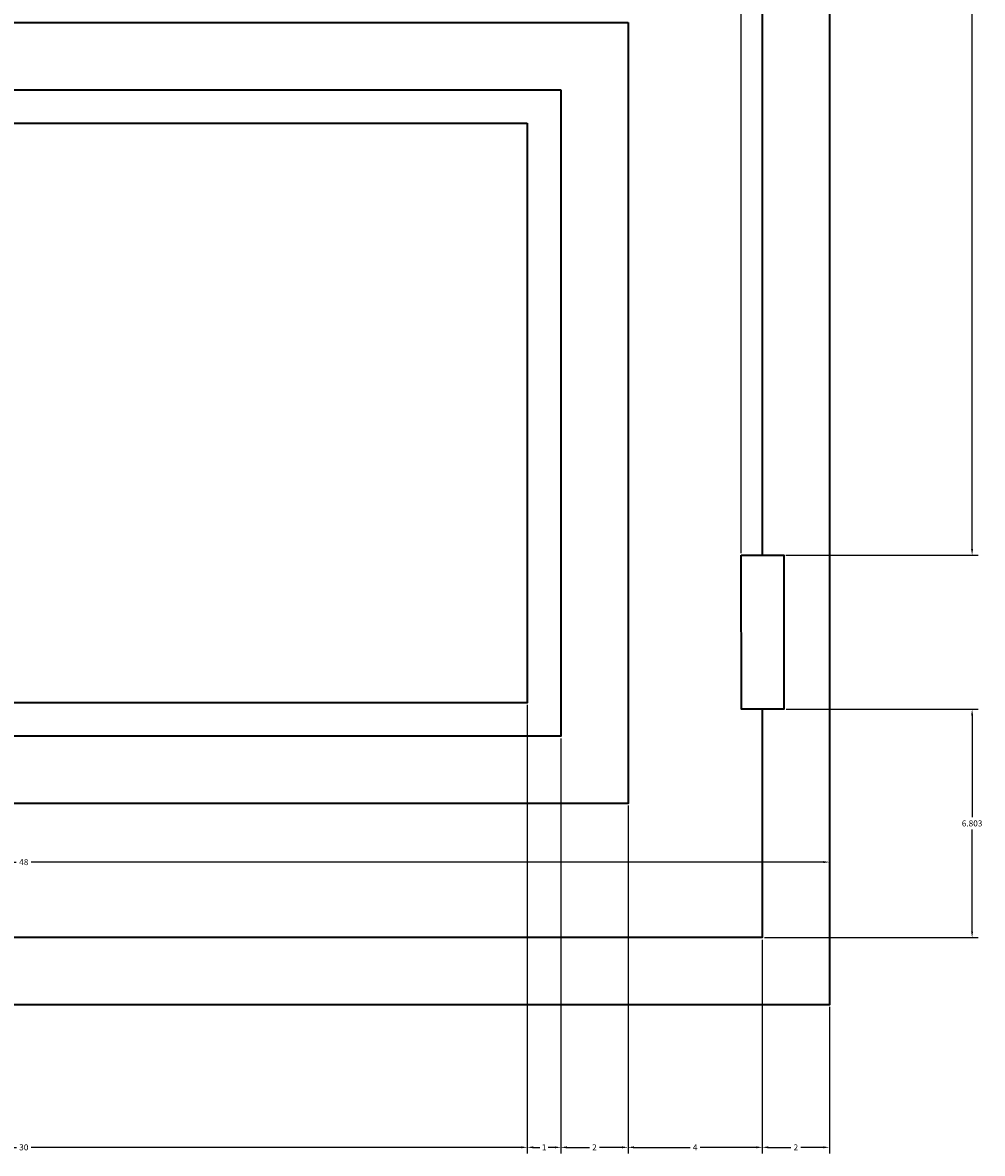
# Model space of a CAD drawing. Units: inches. Extents: x 3137 to 3299, y 1994 to 2089.
# Tile 2 of 14: x 3165 to 3194, y 1994 to 2028. Entities that reach past the tile are written whole.
import ezdxf

# ---------------------------------------------------------------- set-up
doc = ezdxf.new("R2010")
doc.units = ezdxf.units.IN
doc.header["$MEASUREMENT"] = 0
doc.layers.add('A-ANNO-DIMS', color=2, linetype='Continuous', lineweight=18)
doc.layers.add('A-DOOR', color=4, linetype='Continuous', lineweight=35)
doc.styles.get("Standard").update_dxf_attribs({"font": 'arial.ttf'})
doc.dimstyles.get("Standard").update_dxf_attribs({"dimtxt": 0.18, "dimasz": 0.18, "dimexe": 0.18, "dimexo": 0.0625, "dimgap": 0.09, "dimtad": 0, "dimtih": 1, "dimtoh": 1, "dimdec": 4, "dimzin": 0, "dimdsep": 46, "dimtxsty": 'Standard', "dimcen": 0.09, "dimadec": 0, "dimazin": 0, "dimtfac": 1, "dimtdec": 4, "dimtofl": 0, "dimtmove": 0, "dimatfit": 3, "dimfxl": 1, "dimtolj": 1, "dimtzin": 0, "dimarcsym": 0})

# ---------------------------------------------------------------- blocks, each defined once
blk = doc.blocks.new('DOOR-HINGE')
blk.add_lwpolyline([(0, 4.592), (1.268, 4.592), (1.275, 0), (0.007, 0)], close=True)
blk = doc.blocks.new('*D13')
at = {"layer": 'A-ANNO-DIMS', "color": 0, "lineweight": -2, "transparency": 16777216}
for p, q in [((3141.478, 1998.936), (3141.478, 2003.304)), ((3141.658, 2003.124), (3165.255, 2003.124)), ((3189.298, 2003.124), (3165.7, 2003.124)), ((3189.478, 1998.936), (3189.478, 2003.304))]:
    blk.add_line(p, q, dxfattribs=at)
at = {"layer": 'A-ANNO-DIMS', "color": 0, "transparency": 16777216}
for points in [[(3141.658, 2003.154), (3141.658, 2003.094), (3141.478, 2003.124)], [(3189.298, 2003.154), (3189.298, 2003.094), (3189.478, 2003.124)]]:
    blk.add_solid(points, dxfattribs=at)
at = {"layer": 'Defpoints', "color": 0, "transparency": 16777216}
for p in [(3189.478, 2003.124), (3141.478, 1998.874), (3189.478, 1998.874)]:
    blk.add_point(p, dxfattribs=at)
at = {"layer": 'A-ANNO-DIMS', "color": 0, "transparency": 16777216, "insert": (3165.478, 2003.124), "char_height": 0.18, "attachment_point": 5}
blk.add_mtext('\\A1;48', dxfattribs=at)
blk = doc.blocks.new('*D18')
at = {"layer": 'A-ANNO-DIMS', "color": 0, "lineweight": -2, "transparency": 16777216}
for p, q in [((3150.478, 2007.811), (3150.478, 1994.444)), ((3180.478, 2007.811), (3180.478, 1994.444)), ((3150.658, 1994.624), (3165.259, 1994.624)), ((3180.298, 1994.624), (3165.696, 1994.624))]:
    blk.add_line(p, q, dxfattribs=at)
at = {"layer": 'A-ANNO-DIMS', "color": 0, "transparency": 16777216}
for points in [[(3150.658, 1994.654), (3150.658, 1994.594), (3150.478, 1994.624)], [(3180.298, 1994.654), (3180.298, 1994.594), (3180.478, 1994.624)]]:
    blk.add_solid(points, dxfattribs=at)
at = {"layer": 'Defpoints', "color": 0, "transparency": 16777216}
for p in [(3150.478, 2007.874), (3180.478, 2007.874), (3180.478, 1994.624)]:
    blk.add_point(p, dxfattribs=at)
at = {"layer": 'A-ANNO-DIMS', "color": 0, "transparency": 16777216, "insert": (3165.478, 1994.624), "char_height": 0.18, "attachment_point": 5}
blk.add_mtext('\\A1;30', dxfattribs=at)
blk = doc.blocks.new('*D19')
at = {"layer": 'A-ANNO-DIMS', "color": 0, "lineweight": -2, "transparency": 16777216}
for p, q in [((3180.478, 2007.811), (3180.478, 1994.444)), ((3181.478, 2006.811), (3181.478, 1994.444)), ((3180.658, 1994.624), (3180.855, 1994.624)), ((3181.298, 1994.624), (3181.101, 1994.624))]:
    blk.add_line(p, q, dxfattribs=at)
at = {"layer": 'A-ANNO-DIMS', "color": 0, "transparency": 16777216}
for points in [[(3180.658, 1994.654), (3180.658, 1994.594), (3180.478, 1994.624)], [(3181.298, 1994.654), (3181.298, 1994.594), (3181.478, 1994.624)]]:
    blk.add_solid(points, dxfattribs=at)
at = {"layer": 'Defpoints', "color": 0, "transparency": 16777216}
for p in [(3180.478, 2007.874), (3181.478, 2006.874), (3181.478, 1994.624)]:
    blk.add_point(p, dxfattribs=at)
at = {"layer": 'A-ANNO-DIMS', "color": 0, "transparency": 16777216, "insert": (3180.978, 1994.624), "char_height": 0.18, "attachment_point": 5}
blk.add_mtext('\\A1;1', dxfattribs=at)
blk = doc.blocks.new('*D20')
at = {"layer": 'A-ANNO-DIMS', "color": 0, "lineweight": -2, "transparency": 16777216}
for p, q in [((3181.478, 2006.811), (3181.478, 1994.444)), ((3183.478, 2004.811), (3183.478, 1994.444)), ((3181.658, 1994.624), (3182.328, 1994.624)), ((3183.298, 1994.624), (3182.627, 1994.624))]:
    blk.add_line(p, q, dxfattribs=at)
at = {"layer": 'A-ANNO-DIMS', "color": 0, "transparency": 16777216}
for points in [[(3181.658, 1994.654), (3181.658, 1994.594), (3181.478, 1994.624)], [(3183.298, 1994.654), (3183.298, 1994.594), (3183.478, 1994.624)]]:
    blk.add_solid(points, dxfattribs=at)
at = {"layer": 'Defpoints', "color": 0, "transparency": 16777216}
for p in [(3181.478, 2006.874), (3183.478, 2004.874), (3183.478, 1994.624)]:
    blk.add_point(p, dxfattribs=at)
at = {"layer": 'A-ANNO-DIMS', "color": 0, "transparency": 16777216, "insert": (3182.478, 1994.624), "char_height": 0.18, "attachment_point": 5}
blk.add_mtext('\\A1;2', dxfattribs=at)
blk = doc.blocks.new('*D21')
at = {"layer": 'A-ANNO-DIMS', "color": 0, "lineweight": -2, "transparency": 16777216}
for p, q in [((3183.478, 2004.811), (3183.478, 1994.444)), ((3187.478, 2000.811), (3187.478, 1994.444)), ((3183.658, 1994.624), (3185.325, 1994.624)), ((3187.298, 1994.624), (3185.63, 1994.624))]:
    blk.add_line(p, q, dxfattribs=at)
at = {"layer": 'A-ANNO-DIMS', "color": 0, "transparency": 16777216}
for points in [[(3183.658, 1994.654), (3183.658, 1994.594), (3183.478, 1994.624)], [(3187.298, 1994.654), (3187.298, 1994.594), (3187.478, 1994.624)]]:
    blk.add_solid(points, dxfattribs=at)
at = {"layer": 'Defpoints', "color": 0, "transparency": 16777216}
for p in [(3183.478, 2004.874), (3187.478, 2000.874), (3187.478, 1994.624)]:
    blk.add_point(p, dxfattribs=at)
at = {"layer": 'A-ANNO-DIMS', "color": 0, "transparency": 16777216, "insert": (3185.478, 1994.624), "char_height": 0.18, "attachment_point": 5}
blk.add_mtext('\\A1;4', dxfattribs=at)
blk = doc.blocks.new('*D22')
at = {"layer": 'A-ANNO-DIMS', "color": 0, "lineweight": -2, "transparency": 16777216}
for p, q in [((3187.478, 2000.811), (3187.478, 1994.444)), ((3189.478, 1998.811), (3189.478, 1994.444)), ((3187.658, 1994.624), (3188.328, 1994.624)), ((3189.298, 1994.624), (3188.627, 1994.624))]:
    blk.add_line(p, q, dxfattribs=at)
at = {"layer": 'A-ANNO-DIMS', "color": 0, "transparency": 16777216}
for points in [[(3187.658, 1994.654), (3187.658, 1994.594), (3187.478, 1994.624)], [(3189.298, 1994.654), (3189.298, 1994.594), (3189.478, 1994.624)]]:
    blk.add_solid(points, dxfattribs=at)
at = {"layer": 'Defpoints', "color": 0, "transparency": 16777216}
for p in [(3187.478, 2000.874), (3189.478, 1998.874), (3189.478, 1994.624)]:
    blk.add_point(p, dxfattribs=at)
at = {"layer": 'A-ANNO-DIMS', "color": 0, "transparency": 16777216, "insert": (3188.478, 1994.624), "char_height": 0.18, "attachment_point": 5}
blk.add_mtext('\\A1;2', dxfattribs=at)
blk = doc.blocks.new('*D51')
at = {"layer": 'A-ANNO-DIMS', "color": 0, "lineweight": -2, "transparency": 16777216}
for p, q in [((3188.186, 2007.677), (3193.908, 2007.677)), ((3193.728, 2007.497), (3193.728, 2004.458)), ((3193.728, 2001.054), (3193.728, 2004.094)), ((3187.54, 2000.874), (3193.908, 2000.874))]:
    blk.add_line(p, q, dxfattribs=at)
at = {"layer": 'A-ANNO-DIMS', "color": 0, "transparency": 16777216}
for points in [[(3193.698, 2007.497), (3193.758, 2007.497), (3193.728, 2007.677)], [(3193.698, 2001.054), (3193.758, 2001.054), (3193.728, 2000.874)]]:
    blk.add_solid(points, dxfattribs=at)
at = {"layer": 'Defpoints', "color": 0, "transparency": 16777216}
for p in [(3188.124, 2007.677), (3193.728, 2007.677), (3187.478, 2000.874)]:
    blk.add_point(p, dxfattribs=at)
at = {"layer": 'A-ANNO-DIMS', "color": 0, "transparency": 16777216, "insert": (3193.728, 2004.276), "char_height": 0.18, "attachment_point": 5}
blk.add_mtext('\\A1;6.803', dxfattribs=at)
blk = doc.blocks.new('*D52')
at = {"layer": 'A-ANNO-DIMS', "color": 0, "lineweight": -2, "transparency": 16777216}
for p, q in [((3188.174, 2051.649), (3193.908, 2051.649)), ((3193.728, 2051.469), (3193.728, 2032.141)), ((3193.728, 2012.449), (3193.728, 2031.777)), ((3188.18, 2012.269), (3193.908, 2012.269))]:
    blk.add_line(p, q, dxfattribs=at)
at = {"layer": 'A-ANNO-DIMS', "color": 0, "transparency": 16777216}
for points in [[(3193.698, 2051.469), (3193.758, 2051.469), (3193.728, 2051.649)], [(3193.698, 2012.449), (3193.758, 2012.449), (3193.728, 2012.269)]]:
    blk.add_solid(points, dxfattribs=at)
at = {"layer": 'Defpoints', "color": 0, "transparency": 16777216}
for p in [(3188.112, 2051.649), (3193.728, 2051.649), (3188.117, 2012.269)]:
    blk.add_point(p, dxfattribs=at)
at = {"layer": 'A-ANNO-DIMS', "color": 0, "transparency": 16777216, "insert": (3193.728, 2031.959), "char_height": 0.18, "attachment_point": 5}
blk.add_mtext('\\A1;39.38', dxfattribs=at)
blk = doc.blocks.new('*D76')
at = {"layer": 'A-ANNO-DIMS', "color": 0, "lineweight": -2, "transparency": 16777216}
for p, q in [((3186.849, 2012.332), (3186.849, 2087.304)), ((3187.029, 2087.124), (3187.298, 2087.124)), ((3187.478, 2012.332), (3187.478, 2087.304)), ((3187.478, 2087.124), (3187.658, 2087.124))]:
    blk.add_line(p, q, dxfattribs=at)
at = {"layer": 'A-ANNO-DIMS', "color": 0, "transparency": 16777216}
for points in [[(3187.029, 2087.154), (3187.029, 2087.094), (3186.849, 2087.124)], [(3187.298, 2087.154), (3187.298, 2087.094), (3187.478, 2087.124)]]:
    blk.add_solid(points, dxfattribs=at)
at = {"layer": 'Defpoints', "color": 0, "transparency": 16777216}
for p in [(3187.478, 2087.124), (3186.849, 2012.269), (3187.478, 2012.269)]:
    blk.add_point(p, dxfattribs=at)
at = {"layer": 'A-ANNO-DIMS', "color": 0, "transparency": 16777216, "insert": (3188.052, 2087.124), "char_height": 0.18, "attachment_point": 5}
blk.add_mtext('\\A1;0.628', dxfattribs=at)

msp = doc.modelspace()

# ---------------------------------------------------------------- linework, layer by layer
at = {"layer": 'A-DOOR'}
for points in [[(3141.4777, 2082.874), (3189.4777, 2082.874), (3189.4777, 1998.874), (3141.4777, 1998.874)], [(3183.4777, 2028.1375), (3183.4777, 2004.874), (3147.4777, 2004.874), (3147.4777, 2028.1375)], [(3181.4777, 2026.1375), (3181.4777, 2006.874), (3149.4777, 2006.874), (3149.4777, 2026.1375)], [(3180.4777, 2025.1375), (3180.4777, 2007.874), (3150.4777, 2007.874), (3150.4777, 2025.1375)]]:
    msp.add_lwpolyline(points, close=True, dxfattribs=at)
for points in [[(3187.4777, 2007.6773), (3187.4777, 2000.874), (3143.4777, 2000.874), (3143.4777, 2080.874), (3187.4777, 2080.874), (3187.4777, 2076.298)], [(3187.4777, 2051.6494), (3187.4777, 2012.2692)]]:
    msp.add_lwpolyline(points, dxfattribs=at)

# ---------------------------------------------------------------- block references
msp.add_blockref('DOOR-HINGE', (3186.849, 2007.6772), dxfattribs=at)

# ---------------------------------------------------------------- dimensions: what is measured, and where the dimension line sits
at = {"layer": 'A-ANNO-DIMS'}
for base, p1, p2, override, picture, middle in [((3187.4777, 2087.124), (3186.8495, 2012.2692), (3187.4777, 2012.2692), {"dimdec": 3, "dimlfac": 1, "dimrnd": 0, "dimzin": 0, "dimdsep": 46, "dimlunit": 2}, '*D76', (3188.0516, 2087.124)), ((3180.4777, 1994.624), (3150.4777, 2007.874), (3180.4777, 2007.874), {"dimdec": 0, "dimlfac": 1, "dimrnd": 0, "dimzin": 0, "dimdsep": 46, "dimlunit": 2}, '*D18', (3165.4777, 1994.624)), ((3181.4777, 1994.624), (3180.4777, 2007.874), (3181.4777, 2006.874), {"dimdec": 0, "dimlfac": 1, "dimrnd": 0, "dimzin": 0, "dimdsep": 46, "dimlunit": 2}, '*D19', (3180.9777, 1994.624)), ((3183.4777, 1994.624), (3181.4777, 2006.874), (3183.4777, 2004.874), {"dimdec": 0, "dimlfac": 1, "dimrnd": 0, "dimzin": 0, "dimdsep": 46, "dimlunit": 2}, '*D20', (3182.4777, 1994.624)), ((3187.4777, 1994.624), (3183.4777, 2004.874), (3187.4777, 2000.874), {"dimdec": 0, "dimlfac": 1, "dimrnd": 0, "dimzin": 0, "dimdsep": 46, "dimlunit": 2}, '*D21', (3185.4777, 1994.624)), ((3189.4777, 2003.124), (3141.4777, 1998.874), (3189.4777, 1998.874), {"dimdec": 0, "dimlfac": 1, "dimrnd": 0, "dimzin": 0, "dimdsep": 46, "dimlunit": 2}, '*D13', (3165.4777, 2003.124)), ((3189.4777, 1994.624), (3187.4777, 2000.874), (3189.4777, 1998.874), {"dimdec": 0, "dimlfac": 1, "dimrnd": 0, "dimzin": 0, "dimdsep": 46, "dimlunit": 2}, '*D22', (3188.4777, 1994.624))]:
    dim = msp.add_linear_dim(base=base, p1=p1, p2=p2, dimstyle='Standard', override=override, dxfattribs=at)
    dim.commit()
    dim.dimension.update_dxf_attribs({"geometry": picture, "text_midpoint": middle})
for base, p1, p2, override, picture, middle in [((3193.7277, 2051.6494), (3188.1173, 2012.2692), (3188.1116, 2051.6494), {"dimdec": 2, "dimlfac": 1, "dimrnd": 0, "dimzin": 0, "dimdsep": 46, "dimlunit": 2}, '*D52', (3193.7277, 2031.9593)), ((3193.7277, 2007.6773), (3187.4777, 2000.874), (3188.1236, 2007.6773), {"dimdec": 3, "dimlfac": 1, "dimrnd": 0, "dimzin": 0, "dimdsep": 46, "dimlunit": 2}, '*D51', (3193.7277, 2004.2756))]:
    dim = msp.add_linear_dim(base=base, p1=p1, p2=p2, angle=90, dimstyle='Standard', override=override, dxfattribs=at)
    dim.commit()
    dim.dimension.update_dxf_attribs({"geometry": picture, "text_midpoint": middle})

doc.saveas('drawing.dxf')
